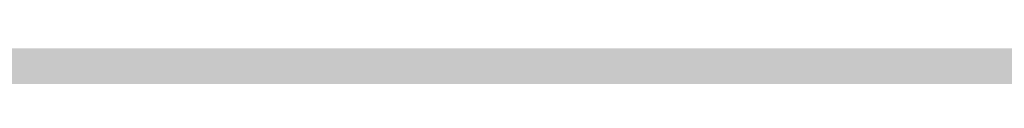
# Model space of a CAD drawing. Units: feet. Extents: x 3168 to 4724, y 827 to 1477.
# Tile 162 of 256: x 3301.4016 to 3301.945, y 1099.0007 to 1099.0148. Entities that reach past the tile are written whole.
import ezdxf

# ---------------------------------------------------------------- set-up
doc = ezdxf.new("R2010")
doc.units = ezdxf.units.FT
doc.layers.add('A-ELEV', color=7, linetype='Continuous', lineweight=35)
doc.layers.add('A-ELEV-PATT', color=8, linetype='Continuous', lineweight=13)

msp = doc.modelspace()

# ---------------------------------------------------------------- hatches: boundary and pattern name
at = {"layer": 'A-ELEV-PATT'}
h = msp.add_hatch(color=256, dxfattribs=at)
h.dxf.hatch_style = 1
edge = h.paths.add_edge_path()
edge.add_ellipse((3552.90576, 979.22014), major_axis=(36.74492, 0), ratio=0.48484848, start_angle=0, end_angle=360)
edge = h.paths.add_edge_path()
edge.add_ellipse((3559.89164, 929.25228), major_axis=(36.74492, 0), ratio=0.48484848, start_angle=0, end_angle=360)
edge = h.paths.add_edge_path()
edge.add_line((3299.31681, 1198.60608), (3479.91671, 1198.60608))
edge.add_line((3479.91671, 1198.60608), (3479.91671, 1209.86857))
edge.add_spline(control_points=[(3479.91671, 1209.86857), (3464.30116, 1209.86857), (3448.6856, 1209.86857), (3410.94914, 1209.86857), (3388.82823, 1209.86857), (3355.64688, 1209.86857), (3344.58642, 1209.86857), (3327.99574, 1209.86857), (3322.46552, 1209.86857), (3314.17018, 1209.86857), (3311.40507, 1209.86857), (3307.2574, 1209.86857), (3305.87484, 1209.86857), (3303.801, 1209.86857), (3303.10973, 1209.86857), (3302.07281, 1209.86857), (3301.72717, 1209.86857), (3301.20871, 1209.86857), (3301.03589, 1209.86857), (3300.77666, 1209.86857), (3300.69025, 1209.86857), (3300.56064, 1209.86857), (3300.51743, 1209.86857), (3300.45263, 1209.86857), (3300.43102, 1209.86857), (3300.39862, 1209.86857), (3300.38782, 1209.86857), (3300.36622, 1209.86857), (3300.34568, 1209.86857), (3300.34555, 1209.86857), (3300.3455, 1209.86857), (3300.3433, 1209.86857), (3300.34115, 1209.86857), (3300.33791, 1209.86857), (3300.33683, 1209.86857), (3300.33394, 1209.86857), (3300.33213, 1209.86857), (3300.32552, 1209.86858), (3300.32071, 1209.86858), (3300.31092, 1209.86859), (3300.30595, 1209.8686), (3300.29051, 1209.86862), (3300.28005, 1209.86865), (3300.23243, 1209.86878), (3300.1953, 1209.86895), (3299.95107, 1209.87061), (3299.74482, 1209.87433), (3299.43683, 1209.88326), (3299.33439, 1209.88679), (3299.18108, 1209.89292), (3299.13003, 1209.8951), (3298.65222, 1209.9168), (3298.22946, 1209.94572), (3297.60163, 1210.00237), (3297.3934, 1210.02346), (3297.08265, 1210.05831), (3296.97933, 1210.07046), (3296.29295, 1210.15486), (3295.71815, 1210.24336), (3294.86872, 1210.39885), (3294.5877, 1210.45448), (3294.16934, 1210.54335), (3294.03042, 1210.57388), (3291.70715, 1211.1012), (3289.65359, 1211.81344), (3285.77626, 1213.56399), (3283.95141, 1214.60348), (3280.51216, 1216.98008), (3278.89724, 1218.31759), (3276.37991, 1220.82949), (3275.41604, 1221.91774), (3274.03934, 1223.7077), (3273.58104, 1224.34953), (3273.14323, 1225.01632)], knot_values=[39.119033, 39.119033, 39.119033, 39.119033, 39.286353, 39.286353, 39.523379, 39.523379, 39.641892, 39.641892, 39.701148, 39.701148, 39.730777, 39.730777, 39.745591, 39.745591, 39.752998, 39.752998, 39.756701, 39.756701, 39.758553, 39.758553, 39.759479, 39.759479, 39.759942, 39.759942, 39.760173, 39.760173, 39.760289, 39.760289, 39.760405, 39.760405, 39.760463, 39.760463, 39.763389, 39.763389, 39.764851, 39.764851, 39.767304, 39.767304, 39.773825, 39.773825, 39.78057, 39.78057, 39.79477, 39.79477, 39.845194, 39.845194, 40.126715, 40.126715, 40.267476, 40.267476, 40.337856, 40.337856, 40.927023, 40.927023, 41.221606, 41.221606, 41.368898, 41.368898, 42.202622, 42.202622, 42.619485, 42.619485, 42.827916, 42.827916, 46.118323, 46.118323, 49.408731, 49.408731, 52.699139, 52.699139, 54.927489, 54.927489, 56.104228, 56.104228, 56.104228, 56.104228], weights=[1, 1, 1, 1, 1, 1, 1, 1, 1, 1, 1, 1, 1, 1, 1, 1, 1, 1, 1, 1, 1, 1, 1, 1, 1, 1, 1, 1, 1, 1, 1, 1, 1, 1, 1, 1, 1, 1, 1, 1, 1, 1, 1, 1, 1, 1, 1, 1, 1, 1, 1, 1, 1, 1, 1, 1, 1, 1, 1, 1, 1, 1, 1, 1, 1, 1, 1, 1, 1, 1, 1, 1, 1, 1], degree=3, periodic=0)
edge.add_line((3273.14323, 1225.01632), (3273.14323, 1099.01632))
edge.add_line((3273.14323, 1099.01632), (3299.31681, 1099.01632))
edge.add_line((3299.31681, 1099.01632), (3299.31681, 1198.60608))
edge = h.paths.add_edge_path()
edge.add_line((3304.75844, 1324.15806), (3479.91671, 1324.15806))
edge.add_line((3479.91671, 1324.15806), (3479.91671, 1335.71462))
edge.add_line((3479.91671, 1335.71462), (3269.16163, 1335.71462))
edge.add_spline(control_points=[(3269.16163, 1335.71462), (3264.02423, 1335.71462), (3258.36412, 1328.95819), (3259.26431, 1323.90027)], knot_values=[0, 0, 0, 0, 15.412191, 15.412191, 15.412191, 15.412191], degree=3, periodic=0)
edge.add_line((3259.26431, 1323.90027), (3265.51685, 1288.76913))
edge.add_line((3265.51685, 1288.76913), (3275.2651, 1261.54563))
edge.add_line((3275.2651, 1261.54563), (3304.75844, 1261.54563))
edge.add_line((3304.75844, 1261.54563), (3304.75844, 1324.15806))
h = msp.add_hatch(color=256, dxfattribs=at)
h.dxf.hatch_style = 1
h.paths.add_polyline_path([(3384.52525, 1099.01632), (3335.02917, 1099.01632), (3299.31681, 1099.01632), (3273.14323, 1099.01632), (3217.56536, 1099.01632), (3168.06928, 827.11626), (3335.02917, 827.11626)])

# ---------------------------------------------------------------- linework, layer by layer
at = {"layer": 'A-ELEV'}
msp.add_open_spline([(3808.5202, 1099.01632), (3808.5202, 1141.41324), (3808.5202, 1183.81015), (3808.5202, 1226.63532), (3808.5202, 1227.06358), (3808.5202, 1227.49183), (3811.49187, 1248.99467), (3814.46354, 1270.49752), (3817.46523, 1292.21756), (3817.49525, 1292.43476), (3817.52526, 1292.65196), (3817.5728, 1310.10675), (3817.62034, 1327.56153), (3817.66788, 1345.01632), (3817.66788, 1345.45796), (3817.66788, 1345.89961), (3817.66788, 1346.45605), (3817.66788, 1346.57084), (3817.66788, 1346.75289), (3817.66788, 1346.82014), (3817.66788, 1346.93487), (3817.66788, 1346.98234), (3817.66788, 1347.03859), (3817.66788, 1347.04736), (3817.66788, 1347.07366), (3817.66788, 1347.0593), (3817.66788, 1347.06155), (3817.66788, 1347.06267), (3817.66788, 1347.06603), (3817.66787, 1347.06827), (3817.66787, 1347.075), (3817.66787, 1347.07949), (3817.66785, 1347.09294), (3817.66783, 1347.1019), (3817.66777, 1347.12879), (3817.6677, 1347.1467), (3817.66743, 1347.20042), (3817.66716, 1347.23619), (3817.6661, 1347.34338), (3817.66504, 1347.41469), (3817.66081, 1347.62809), (3817.65661, 1347.76971), (3817.63997, 1348.19249), (3817.62351, 1348.47159), (3817.55909, 1349.30007), (3817.49612, 1349.84059), (3817.25543, 1351.42416), (3817.02632, 1352.42879), (3816.30687, 1354.88891), (3815.74375, 1356.26873), (3814.46396, 1358.81921), (3813.74641, 1359.99097), (3812.19584, 1362.17234), (3811.36225, 1363.18212), (3809.58884, 1365.06901), (3808.64882, 1365.94611), (3806.65426, 1367.57962), (3805.5997, 1368.33615), (3803.35289, 1369.72233), (3802.16054, 1370.35239), (3799.60081, 1371.45359), (3798.23269, 1371.92548), (3795.28008, 1372.63462), (3793.69315, 1372.87207), (3791.86944, 1372.92648), (3791.74086, 1372.92922), (3791.35337, 1372.9341), (3791.09271, 1372.9329), (3790.30412, 1372.91507), (3789.76954, 1372.88419), (3789.20919, 1372.83024), (3789.19062, 1372.82842), (3789.13489, 1372.82291), (3789.0977, 1372.81914), (3789.04844, 1372.81401), (3789.0364, 1372.81274), (3789.00026, 1372.80892), (3788.97615, 1372.80633), (3788.9494, 1372.8034), (3788.94679, 1372.80312), (3788.94257, 1372.80266), (3788.94097, 1372.80248), (3788.93857, 1372.80222), (3788.93778, 1372.80213), (3788.93539, 1372.80187), (3788.86753, 1372.7944), (3788.75687, 1372.78223), (3788.70153, 1372.77614), (3788.53553, 1372.75788), (3788.42486, 1372.74571), (3788.09286, 1372.70918), (3787.87152, 1372.68484), (3787.20751, 1372.61179), (3786.76483, 1372.5631), (3785.43681, 1372.41701), (3784.55147, 1372.31962), (3781.89542, 1372.02744), (3780.12473, 1371.83266), (3774.81265, 1371.24831), (3771.27126, 1370.85874), (3760.64709, 1369.69004), (3753.56431, 1368.9109), (3732.31597, 1366.5735), (3718.15042, 1365.01523), (3694.00676, 1362.35933), (3684.02866, 1361.26169), (3674.05056, 1360.16406), (3664.60066, 1360.16406), (3655.15077, 1360.16406), (3626.80108, 1360.16406), (3607.90129, 1360.16406), (3551.20192, 1360.16406), (3513.40234, 1360.16406), (3467.72518, 1360.16406), (3459.8476, 1360.16406), (3436.21487, 1360.16406), (3420.45972, 1360.16406), (3373.19425, 1360.16406), (3341.68395, 1360.16406), (3302.84816, 1360.16406), (3295.52269, 1360.16406), (3286.03829, 1360.16406), (3283.87937, 1360.16406), (3277.40261, 1360.16406), (3273.08477, 1360.16406), (3267.73285, 1360.16406), (3266.69877, 1360.16406), (3263.59652, 1360.16406), (3261.52835, 1360.16406), (3259.23694, 1360.16406), (3259.0137, 1360.16406), (3258.34396, 1360.16406), (3257.89747, 1360.16406), (3257.431, 1360.16406), (3257.41102, 1360.16406), (3257.37057, 1360.16406), (3257.37547, 1360.16406), (3257.3746, 1360.16406), (3257.37394, 1360.16406), (3257.37196, 1360.16406), (3257.37064, 1360.16406), (3257.36667, 1360.16406), (3257.36403, 1360.16406), (3257.35611, 1360.16405), (3257.35083, 1360.16405), (3257.33499, 1360.16402), (3257.32443, 1360.164), (3257.29277, 1360.1639), (3257.27168, 1360.1638), (3257.20844, 1360.1634), (3257.16634, 1360.163), (3257.04021, 1360.16139), (3256.95635, 1360.15978), (3256.7055, 1360.15339), (3256.53924, 1360.14704), (3256.04357, 1360.12192), (3255.7173, 1360.0971), (3254.75245, 1360.00048), (3254.12797, 1359.90651), (3252.18007, 1359.52533), (3250.94157, 1359.14399), (3248.67018, 1358.24329), (3247.63574, 1357.72383), (3245.73263, 1356.60347), (3244.86339, 1356.00206), (3243.25311, 1354.74287), (3242.51197, 1354.08473), (3240.75105, 1352.34478), (3239.80096, 1351.22957), (3238.08777, 1348.87244), (3237.32469, 1347.63036), (3235.98251, 1344.97163), (3235.40221, 1343.55491), (3234.59108, 1340.81546), (3234.31088, 1339.54355), (3233.97649, 1336.80256), (3233.92211, 1335.33088), (3234.14892, 1332.59127), (3234.34953, 1331.3672), (3234.71989, 1329.99937), (3234.75242, 1329.88336), (3234.85362, 1329.5348), (3234.92589, 1329.30168), (3235.02484, 1329.00255), (3235.04692, 1328.93693), (3235.07764, 1328.84724), (3235.08592, 1328.8232), (3235.11094, 1328.75106), (3235.12783, 1328.70296), (3235.14799, 1328.64624), (3235.15106, 1328.63763), (3235.1561, 1328.62353), (3235.15806, 1328.61803), (3235.16021, 1328.61203), (3235.16561, 1328.59694), (3235.1801, 1328.55649), (3235.19026, 1328.5281), (3235.22076, 1328.44295), (3235.24108, 1328.38618), (3235.30207, 1328.21587), (3235.34273, 1328.10232), (3235.4647, 1327.7617), (3235.54601, 1327.53462), (3235.78995, 1326.85338), (3235.95258, 1326.39922), (3236.44046, 1325.03674), (3236.76571, 1324.12841), (3237.74148, 1321.40345), (3238.39198, 1319.5868), (3240.34351, 1314.13687), (3241.64452, 1310.50358), (3245.54757, 1299.60371), (3248.14961, 1292.33713), (3255.95571, 1270.53739), (3261.15977, 1256.00423), (3267.38762, 1238.612), (3268.4114, 1235.75294), (3269.51038, 1232.68386), (3269.58558, 1232.47385), (3269.70661, 1232.13585), (3269.75244, 1232.00786), (3269.82733, 1231.79873), (3269.85638, 1231.7176), (3269.90632, 1231.57812), (3269.92721, 1231.51978), (3269.97247, 1231.39341), (3269.99683, 1231.32537), (3270.0265, 1231.24251), (3270.03181, 1231.22768), (3270.04028, 1231.20402), (3270.03922, 1231.20698), (3270.03936, 1231.2066), (3270.03943, 1231.20641), (3270.03963, 1231.20585), (3270.03977, 1231.20547), (3270.04017, 1231.20433), (3270.04044, 1231.20358), (3270.04125, 1231.20131), (3270.0418, 1231.1998), (3270.04342, 1231.19527), (3270.0445, 1231.19225), (3270.04776, 1231.18318), (3270.04993, 1231.17714), (3270.05644, 1231.15903), (3270.06079, 1231.14696), (3270.07387, 1231.11076), (3270.08261, 1231.08666), (3270.10894, 1231.01441), (3270.1266, 1230.96635), (3270.17993, 1230.82246), (3270.21595, 1230.72692), (3270.32532, 1230.44151), (3270.40003, 1230.25281), (3270.62925, 1229.69144), (3270.78888, 1229.3235), (3271.28649, 1228.23832), (3271.6431, 1227.53975), (3272.77586, 1225.51528), (3273.61417, 1224.2605), (3275.41604, 1221.91774), (3276.37991, 1220.82949), (3278.89724, 1218.31759), (3280.51216, 1216.98008), (3283.95141, 1214.60348), (3285.77626, 1213.56399), (3289.65359, 1211.81344), (3291.70715, 1211.1012), (3294.03042, 1210.57388), (3294.16934, 1210.54335), (3294.5877, 1210.45448), (3294.86872, 1210.39885), (3295.71815, 1210.24336), (3296.29295, 1210.15486), (3296.97933, 1210.07046), (3297.08265, 1210.05831), (3297.3934, 1210.02346), (3297.60163, 1210.00237), (3298.22946, 1209.94572), (3298.65222, 1209.9168), (3299.13003, 1209.8951), (3299.18108, 1209.89292), (3299.33439, 1209.88679), (3299.43683, 1209.88326), (3299.74482, 1209.87433), (3299.95107, 1209.87061), (3300.1953, 1209.86895), (3300.23243, 1209.86878), (3300.28005, 1209.86865), (3300.29051, 1209.86862), (3300.30595, 1209.8686), (3300.31092, 1209.86859), (3300.32071, 1209.86858), (3300.32552, 1209.86858), (3300.33213, 1209.86857), (3300.33394, 1209.86857), (3300.33683, 1209.86857), (3300.33791, 1209.86857), (3300.34115, 1209.86857), (3300.3433, 1209.86857), (3300.3455, 1209.86857), (3300.34555, 1209.86857), (3300.34568, 1209.86857), (3300.36622, 1209.86857), (3300.38782, 1209.86857), (3300.39862, 1209.86857), (3300.43102, 1209.86857), (3300.45263, 1209.86857), (3300.51743, 1209.86857), (3300.56064, 1209.86857), (3300.69025, 1209.86857), (3300.77666, 1209.86857), (3301.03589, 1209.86857), (3301.20871, 1209.86857), (3301.72717, 1209.86857), (3302.07281, 1209.86857), (3303.10973, 1209.86857), (3303.801, 1209.86857), (3305.87484, 1209.86857), (3307.2574, 1209.86857), (3311.40507, 1209.86857), (3314.17018, 1209.86857), (3322.46552, 1209.86857), (3327.99574, 1209.86857), (3344.58642, 1209.86857), (3355.64688, 1209.86857), (3388.82823, 1209.86857), (3410.94914, 1209.86857), (3477.31185, 1209.86857), (3521.55366, 1209.86857), (3566.83618, 1209.86857), (3567.87689, 1209.86857), (3570.99902, 1209.86857), (3573.08043, 1209.86857), (3575.7814, 1209.86857), (3576.40094, 1209.86857), (3577.29582, 1209.86857), (3577.57115, 1209.86857), (3578.39715, 1209.86857), (3578.94781, 1209.86857), (3579.75649, 1209.86857), (3580.01451, 1209.86857), (3580.34274, 1209.86857), (3580.32686, 1209.86857), (3580.32717, 1209.86857), (3580.32732, 1209.86857), (3580.32778, 1209.86857), (3580.32809, 1209.86857), (3580.329, 1209.86857), (3580.32961, 1209.86857), (3580.33145, 1209.86857), (3580.33267, 1209.86857), (3580.33633, 1209.86857), (3580.33878, 1209.86857), (3580.34611, 1209.86856), (3580.35099, 1209.86856), (3580.36566, 1209.86854), (3580.37544, 1209.86852), (3580.4048, 1209.86845), (3580.42439, 1209.86838), (3580.48318, 1209.86808), (3580.52244, 1209.86779), (3580.64036, 1209.86662), (3580.71919, 1209.86545), (3580.95632, 1209.86077), (3581.11522, 1209.85607), (3581.59416, 1209.83723), (3581.91642, 1209.81833), (3582.88995, 1209.74243), (3583.54799, 1209.66617), (3585.53183, 1209.36062), (3586.86722, 1209.05389), (3589.47155, 1208.25247), (3590.74024, 1207.75785), (3591.99545, 1207.1588), (3592.05781, 1207.12874), (3592.24424, 1207.03795), (3592.36768, 1206.97663), (3592.73528, 1206.79036), (3592.97675, 1206.6631), (3593.24454, 1206.51644), (3593.27473, 1206.49982), (3593.36512, 1206.44984), (3593.42511, 1206.41633), (3593.60431, 1206.31529), (3593.72273, 1206.24721), (3593.85721, 1206.1684), (3593.87436, 1206.15832), (3593.92574, 1206.12804), (3593.9599, 1206.1078), (3594.06209, 1206.0469), (3594.12983, 1206.00607), (3594.20844, 1205.95817), (3594.21968, 1205.9513), (3594.25339, 1205.93069), (3594.27582, 1205.91692), (3594.34297, 1205.87554), (3594.38756, 1205.84785), (3594.43362, 1205.81905), (3594.43526, 1205.81802), (3594.44017, 1205.81495), (3594.44345, 1205.81289), (3594.44712, 1205.81059), (3594.44752, 1205.81035), (3594.44869, 1205.80961), (3594.44948, 1205.80912), (3594.45037, 1205.80856), (3594.45047, 1205.8085), (3594.4506, 1205.80842), (3594.4674, 1205.79789), (3594.49327, 1205.78167), (3594.5062, 1205.77357), (3594.54501, 1205.74925), (3594.57088, 1205.73303), (3594.64849, 1205.6844), (3594.70023, 1205.65197), (3594.85544, 1205.55469), (3594.95892, 1205.48984), (3595.26936, 1205.29528), (3595.47631, 1205.16558), (3596.09719, 1204.77646), (3596.5111, 1204.51705), (3597.75284, 1203.73883), (3598.58067, 1203.22001), (3601.06415, 1201.66355), (3602.71981, 1200.62591), (3607.68677, 1197.513), (3610.99809, 1195.43773), (3620.93202, 1189.2119), (3627.55464, 1185.06135), (3647.42251, 1172.60971), (3660.66775, 1164.30861), (3700.40348, 1139.40531), (3726.89397, 1122.80312), (3757.20572, 1103.80605), (3761.02697, 1101.41118), (3764.84822, 1099.01632), (3745.32827, 1099.01632), (3725.80832, 1099.01632), (3706.28837, 1099.01632), (3706.28837, 1108.45324), (3706.28837, 1117.89016), (3706.28837, 1127.32708), (3710.75075, 1127.32708), (3715.21314, 1127.32708), (3719.67553, 1127.32708)], degree=3, knots=[0, 0, 0, 0, 0.982037, 0.982037, 0.991957, 0.991957, 0.991957, 1.966522, 1.966522, 1.976367, 1.976367, 1.976367, 2.976367, 2.976367, 2.976367, 3.00169, 3.00169, 3.008272, 3.008272, 3.012129, 3.012129, 3.014851, 3.014851, 3.015353, 3.015353, 3.016359, 3.016359, 3.017365, 3.017365, 3.019376, 3.019376, 3.023398, 3.023398, 3.031442, 3.031442, 3.047531, 3.047531, 3.079708, 3.079708, 3.144063, 3.144063, 3.272772, 3.272772, 3.53019, 3.53019, 4.045026, 4.045026, 5.074698, 5.074698, 6.700878, 6.700878, 8.327058, 8.327058, 9.953238, 9.953238, 11.579418, 11.579418, 13.205598, 13.205598, 14.831778, 14.831778, 16.457958, 16.457958, 18.084138, 18.084138, 18.206872, 18.206872, 18.45234, 18.45234, 18.943275, 18.943275, 18.960093, 18.960093, 18.993729, 18.993729, 19.00461, 19.00461, 19.026374, 19.026374, 19.028737, 19.028737, 19.03018, 19.03018, 19.030897, 19.030897, 19.032332, 19.032332, 19.033766, 19.033766, 19.036636, 19.036636, 19.042374, 19.042374, 19.053851, 19.053851, 19.076805, 19.076805, 19.122714, 19.122714, 19.21453, 19.21453, 19.398163, 19.398163, 19.765429, 19.765429, 20.024128, 20.024128, 20.024128, 20.092031, 20.092031, 20.227836, 20.227836, 20.499446, 20.499446, 20.556051, 20.556051, 20.66926, 20.66926, 20.895678, 20.895678, 20.948316, 20.948316, 20.963829, 20.963829, 20.994855, 20.994855, 21.002285, 21.002285, 21.017146, 21.017146, 21.01875, 21.01875, 21.021959, 21.021959, 21.022102, 21.022102, 21.022249, 21.022249, 21.022708, 21.022708, 21.023627, 21.023627, 21.025464, 21.025464, 21.029138, 21.029138, 21.036486, 21.036486, 21.051183, 21.051183, 21.080575, 21.080575, 21.139361, 21.139361, 21.256932, 21.256932, 21.492073, 21.492073, 21.962356, 21.962356, 23.01002, 23.01002, 24.057684, 24.057684, 25.105348, 25.105348, 26.153011, 26.153011, 27.776787, 27.776787, 29.400562, 29.400562, 31.024337, 31.024337, 32.278801, 32.278801, 33.533265, 33.533265, 34.467568, 34.467568, 34.553971, 34.553971, 34.726776, 34.726776, 34.775309, 34.775309, 34.793079, 34.793079, 34.82862, 34.82862, 34.834979, 34.834979, 34.839039, 34.839039, 34.839411, 34.839411, 34.840285, 34.840285, 34.842034, 34.842034, 34.845531, 34.845531, 34.852525, 34.852525, 34.866512, 34.866512, 34.894488, 34.894488, 34.950439, 34.950439, 35.062342, 35.062342, 35.286147, 35.286147, 35.733758, 35.733758, 35.821815, 35.821815, 35.828283, 35.828283, 35.832225, 35.832225, 35.834724, 35.834724, 35.836521, 35.836521, 35.838617, 35.838617, 35.839073, 35.839073, 35.839345, 35.839345, 35.839617, 35.839617, 35.840161, 35.840161, 35.841249, 35.841249, 35.843425, 35.843425, 35.847778, 35.847778, 35.856482, 35.856482, 35.873891, 35.873891, 35.908709, 35.908709, 35.978345, 35.978345, 36.117617, 36.117617, 36.396161, 36.396161, 36.953248, 36.953248, 38.067423, 38.067423, 40.295772, 40.295772, 42.524122, 42.524122, 45.81453, 45.81453, 49.104937, 49.104937, 52.395345, 52.395345, 52.603776, 52.603776, 53.020639, 53.020639, 53.854363, 53.854363, 54.001655, 54.001655, 54.296238, 54.296238, 54.885405, 54.885405, 54.955785, 54.955785, 55.096546, 55.096546, 55.378067, 55.378067, 55.42849, 55.42849, 55.442691, 55.442691, 55.449436, 55.449436, 55.455957, 55.455957, 55.458409, 55.458409, 55.459872, 55.459872, 55.462798, 55.462798, 55.462856, 55.462856, 55.462972, 55.462972, 55.463088, 55.463088, 55.463319, 55.463319, 55.463782, 55.463782, 55.464708, 55.464708, 55.46656, 55.46656, 55.470263, 55.470263, 55.47767, 55.47767, 55.492484, 55.492484, 55.522112, 55.522112, 55.581369, 55.581369, 55.699882, 55.699882, 55.936907, 55.936907, 56.410959, 56.410959, 56.42211, 56.42211, 56.444413, 56.444413, 56.451051, 56.451051, 56.454001, 56.454001, 56.459901, 56.459901, 56.462666, 56.462666, 56.463418, 56.463418, 56.464171, 56.464171, 56.465675, 56.465675, 56.468684, 56.468684, 56.474702, 56.474702, 56.486738, 56.486738, 56.51081, 56.51081, 56.558955, 56.558955, 56.655243, 56.655243, 56.847821, 56.847821, 57.232975, 57.232975, 58.003284, 58.003284, 59.543901, 59.543901, 62.625137, 62.625137, 68.787607, 68.787607, 74.950078, 74.950078, 75.27336, 75.27336, 75.919923, 75.919923, 77.213051, 77.213051, 77.377769, 77.377769, 77.707206, 77.707206, 78.366079, 78.366079, 78.462532, 78.462532, 78.655436, 78.655436, 79.041245, 79.041245, 79.105735, 79.105735, 79.234714, 79.234714, 79.492672, 79.492672, 79.502197, 79.502197, 79.521249, 79.521249, 79.523534, 79.523534, 79.528103, 79.528103, 79.528682, 79.528682, 79.528885, 79.528885, 79.529089, 79.529089, 79.529495, 79.529495, 79.530308, 79.530308, 79.531935, 79.531935, 79.535187, 79.535187, 79.541693, 79.541693, 79.554704, 79.554704, 79.580725, 79.580725, 79.632769, 79.632769, 79.736856, 79.736856, 79.94503, 79.94503, 80.361377, 80.361377, 80.421435, 80.421435, 80.421435, 81.421435, 81.421435, 81.421435, 82.421435, 82.421435, 82.421435, 83.421435, 83.421435, 83.421435, 83.421435], dxfattribs=at)

doc.saveas('drawing.dxf')
